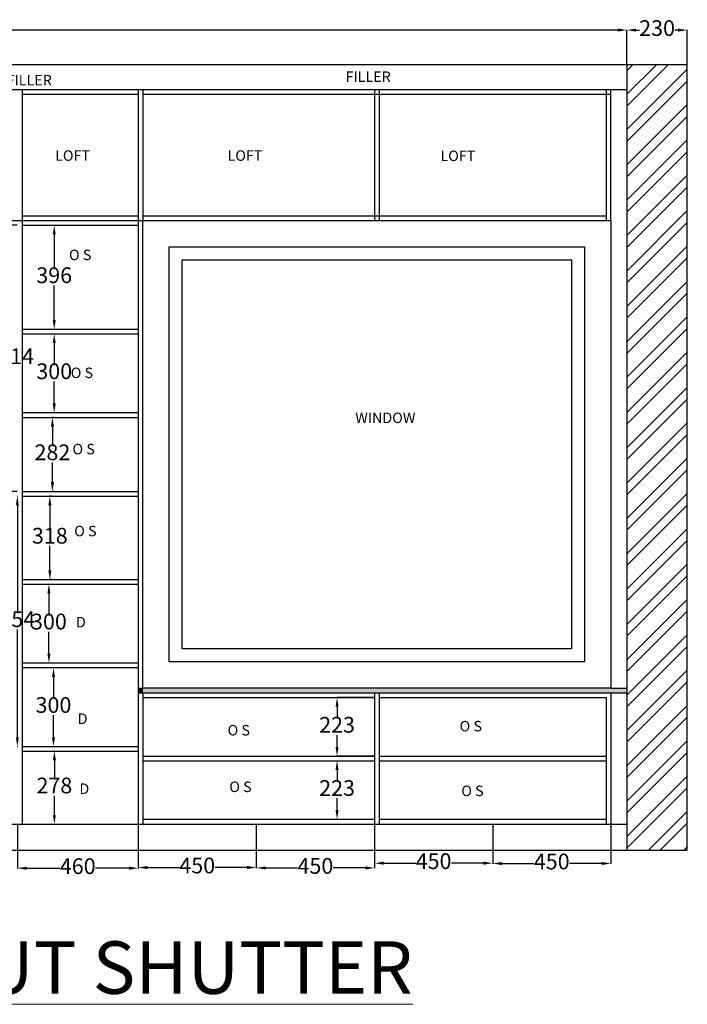
# Model space of a CAD drawing. Units: millimetres. Extents: x 1304 to 14372, y 283 to 7516.
# Tile 3 of 4: x 5077 to 7619, y 283 to 4036. Entities that reach past the tile are written whole.
import ezdxf

# ---------------------------------------------------------------- set-up
doc = ezdxf.new("R2010")
doc.units = ezdxf.units.MM
doc.layers.get('Defpoints').update_dxf_attribs({"color": 2})
for name, color, linetype, lineweight in [('A-ANNO-DIMS', 2, 'Continuous', 18), ('A-ANNO-TEXT', 3, 'Continuous', 18), ('A-FURN', 7, 'Continuous', 25), ('A-FURN-PATT', 8, 'Continuous', 13)]:
    doc.layers.add(name, color=color, linetype=linetype, lineweight=lineweight)
doc.styles.get("Standard").update_dxf_attribs({"font": 'arial.ttf'})
doc.dimstyles.new('ISO-25', dxfattribs={"dimtxt": 60, "dimasz": 35, "dimexe": 1.25, "dimexo": 0.625, "dimtad": 0, "dimtih": 1, "dimtoh": 1, "dimtxsty": 'Standard', "dimcen": 2.5, "dimclrd": 1, "dimclre": 3, "dimadec": 0, "dimazin": 0, "dimtfac": 1, "dimtmove": 0, "dimatfit": 3, "dimfxl": 1, "dimarcsym": 0})

# ---------------------------------------------------------------- blocks, each defined once
blk = doc.blocks.new('*D16')
at = {"layer": 'A-ANNO-DIMS', "color": 0, "lineweight": -2, "transparency": 16777216}
for p, q in [((2248.6, 4008), (2248.6, 3995.4)), ((2283.6, 3996.6), (4728.5, 3996.6)), ((7353.6, 3996.6), (4908.8, 3996.6)), ((7388.6, 3865.9), (7388.6, 3997.9))]:
    blk.add_line(p, q, dxfattribs=at)
at = {"layer": 'A-ANNO-DIMS', "color": 0, "transparency": 16777216}
for points in [[(2283.6, 4002.4), (2283.6, 3990.8), (2248.6, 3996.6)], [(7353.6, 4002.4), (7353.6, 3990.8), (7388.6, 3996.6)]]:
    blk.add_solid(points, dxfattribs=at)
at = {"layer": 'Defpoints', "color": 0, "transparency": 16777216}
for p in [(2248.6, 4008.6), (7388.6, 3996.6), (7388.6, 3865.3)]:
    blk.add_point(p, dxfattribs=at)
at = {"layer": 'A-ANNO-DIMS', "color": 0, "transparency": 16777216, "insert": (4818.6, 3996.6), "char_height": 60, "attachment_point": 5}
blk.add_mtext('5140', dxfattribs=at)
blk = doc.blocks.new('*D17')
at = {"layer": 'A-ANNO-DIMS', "color": 0, "lineweight": -2, "transparency": 16777216}
for p, q in [((7388.6, 3865.9), (7388.6, 3997.5)), ((7423.6, 3996.3), (7436.3, 3996.3)), ((7583.6, 3996.3), (7571, 3996.3)), ((7618.6, 3865.9), (7618.6, 3997.5))]:
    blk.add_line(p, q, dxfattribs=at)
at = {"layer": 'A-ANNO-DIMS', "color": 0, "transparency": 16777216}
for points in [[(7423.6, 4002.1), (7423.6, 3990.4), (7388.6, 3996.3)], [(7583.6, 4002.1), (7583.6, 3990.4), (7618.6, 3996.3)]]:
    blk.add_solid(points, dxfattribs=at)
at = {"layer": 'Defpoints', "color": 0, "transparency": 16777216}
for p in [(7618.6, 3996.3), (7388.6, 3865.3), (7618.6, 3865.3)]:
    blk.add_point(p, dxfattribs=at)
at = {"layer": 'A-ANNO-DIMS', "color": 0, "transparency": 16777216, "insert": (7503.6, 3996.3), "char_height": 60, "attachment_point": 5}
blk.add_mtext('230', dxfattribs=at)
blk = doc.blocks.new('*D23')
at = {"layer": 'A-ANNO-DIMS', "color": 0, "lineweight": -2, "transparency": 16777216}
for p, q in [((5067, 3252.3), (5038.8, 3252.3)), ((5040.1, 3217.3), (5040.1, 2776.5)), ((5040.1, 2273.3), (5040.1, 2714)), ((5067, 2238.3), (5038.8, 2238.3))]:
    blk.add_line(p, q, dxfattribs=at)
at = {"layer": 'A-ANNO-DIMS', "color": 0, "transparency": 16777216}
for points in [[(5034.2, 3217.3), (5045.9, 3217.3), (5040.1, 3252.3)], [(5034.2, 2273.3), (5045.9, 2273.3), (5040.1, 2238.3)]]:
    blk.add_solid(points, dxfattribs=at)
at = {"layer": 'Defpoints', "color": 0, "transparency": 16777216}
for p in [(5067.6, 3252.3), (5040.1, 2238.3), (5067.6, 2238.3)]:
    blk.add_point(p, dxfattribs=at)
at = {"layer": 'A-ANNO-DIMS', "color": 0, "transparency": 16777216, "insert": (5040.1, 2745.3), "char_height": 60, "attachment_point": 5}
blk.add_mtext('1014', dxfattribs=at)
blk = doc.blocks.new('*D24')
at = {"layer": 'A-ANNO-DIMS', "color": 0, "lineweight": -2, "transparency": 16777216}
for p, q in [((5068.3, 2220.3), (5068.9, 2220.3)), ((5067.6, 2185.3), (5067.6, 1774.5)), ((5067.6, 1301.3), (5067.6, 1712)), ((5068.3, 1266.3), (5068.9, 1266.3))]:
    blk.add_line(p, q, dxfattribs=at)
at = {"layer": 'A-ANNO-DIMS', "color": 0, "transparency": 16777216}
for points in [[(5061.8, 2185.3), (5073.5, 2185.3), (5067.6, 2220.3)], [(5061.8, 1301.3), (5073.5, 1301.3), (5067.6, 1266.3)]]:
    blk.add_solid(points, dxfattribs=at)
at = {"layer": 'Defpoints', "color": 0, "transparency": 16777216}
for p in [(5067.6, 2220.3), (5067.6, 1266.3), (5067.6, 1266.3)]:
    blk.add_point(p, dxfattribs=at)
at = {"layer": 'A-ANNO-DIMS', "color": 0, "transparency": 16777216, "insert": (5067.6, 1743.3), "char_height": 60, "attachment_point": 5}
blk.add_mtext('954', dxfattribs=at)
blk = doc.blocks.new('*D25')
at = {"layer": 'A-ANNO-DIMS', "color": 0, "lineweight": -2, "transparency": 16777216}
for p, q in [((5086.3, 3252.3), (5209.4, 3252.3)), ((5208.1, 3217.3), (5208.1, 3085.6)), ((5208.1, 2891.3), (5208.1, 3023)), ((5086.3, 2856.3), (5209.4, 2856.3))]:
    blk.add_line(p, q, dxfattribs=at)
at = {"layer": 'A-ANNO-DIMS', "color": 0, "transparency": 16777216}
for points in [[(5202.3, 3217.3), (5213.9, 3217.3), (5208.1, 3252.3)], [(5202.3, 2891.3), (5213.9, 2891.3), (5208.1, 2856.3)]]:
    blk.add_solid(points, dxfattribs=at)
at = {"layer": 'Defpoints', "color": 0, "transparency": 16777216}
for p in [(5085.6, 3252.3), (5085.6, 2856.3), (5208.1, 2856.3)]:
    blk.add_point(p, dxfattribs=at)
at = {"layer": 'A-ANNO-DIMS', "color": 0, "transparency": 16777216, "insert": (5208.1, 3054.3), "char_height": 60, "attachment_point": 5}
blk.add_mtext('396', dxfattribs=at)
blk = doc.blocks.new('*D26')
at = {"layer": 'A-ANNO-DIMS', "color": 0, "lineweight": -2, "transparency": 16777216}
for p, q in [((5208.7, 2838.3), (5209.4, 2838.3)), ((5208.1, 2803.3), (5208.1, 2719.6)), ((5208.1, 2573.3), (5208.1, 2657)), ((5208.7, 2538.3), (5209.4, 2538.3))]:
    blk.add_line(p, q, dxfattribs=at)
at = {"layer": 'A-ANNO-DIMS', "color": 0, "transparency": 16777216}
for points in [[(5202.3, 2803.3), (5213.9, 2803.3), (5208.1, 2838.3)], [(5202.3, 2573.3), (5213.9, 2573.3), (5208.1, 2538.3)]]:
    blk.add_solid(points, dxfattribs=at)
at = {"layer": 'Defpoints', "color": 0, "transparency": 16777216}
for p in [(5208.1, 2838.3), (5208.1, 2538.3), (5208.1, 2538.3)]:
    blk.add_point(p, dxfattribs=at)
at = {"layer": 'A-ANNO-DIMS', "color": 0, "transparency": 16777216, "insert": (5208.1, 2688.3), "char_height": 60, "attachment_point": 5}
blk.add_mtext('300', dxfattribs=at)
blk = doc.blocks.new('*D27')
at = {"layer": 'A-ANNO-DIMS', "color": 0, "lineweight": -2, "transparency": 16777216}
for p, q in [((5207.5, 2520.3), (5199.9, 2520.3)), ((5201.2, 2485.3), (5201.2, 2410.5)), ((5201.2, 2273.3), (5201.2, 2348)), ((5207.5, 2238.3), (5199.9, 2238.3))]:
    blk.add_line(p, q, dxfattribs=at)
at = {"layer": 'A-ANNO-DIMS', "color": 0, "transparency": 16777216}
for points in [[(5195.4, 2485.3), (5207, 2485.3), (5201.2, 2520.3)], [(5195.4, 2273.3), (5207, 2273.3), (5201.2, 2238.3)]]:
    blk.add_solid(points, dxfattribs=at)
at = {"layer": 'Defpoints', "color": 0, "transparency": 16777216}
for p in [(5208.1, 2520.3), (5201.2, 2238.3), (5208.1, 2238.3)]:
    blk.add_point(p, dxfattribs=at)
at = {"layer": 'A-ANNO-DIMS', "color": 0, "transparency": 16777216, "insert": (5201.2, 2379.3), "char_height": 60, "attachment_point": 5}
blk.add_mtext('282', dxfattribs=at)
blk = doc.blocks.new('*D28')
at = {"layer": 'A-ANNO-DIMS', "color": 0, "lineweight": -2, "transparency": 16777216}
for p, q in [((5200.6, 2220.3), (5190.2, 2220.3)), ((5191.4, 2185.3), (5191.4, 2092.6)), ((5191.4, 1937.3), (5191.4, 2030)), ((5200.6, 1902.3), (5190.2, 1902.3))]:
    blk.add_line(p, q, dxfattribs=at)
at = {"layer": 'A-ANNO-DIMS', "color": 0, "transparency": 16777216}
for points in [[(5185.6, 2185.3), (5197.3, 2185.3), (5191.4, 2220.3)], [(5185.6, 1937.3), (5197.3, 1937.3), (5191.4, 1902.3)]]:
    blk.add_solid(points, dxfattribs=at)
at = {"layer": 'Defpoints', "color": 0, "transparency": 16777216}
for p in [(5201.2, 2220.3), (5191.4, 1902.3), (5201.2, 1902.3)]:
    blk.add_point(p, dxfattribs=at)
at = {"layer": 'A-ANNO-DIMS', "color": 0, "transparency": 16777216, "insert": (5191.4, 2061.3), "char_height": 60, "attachment_point": 5}
blk.add_mtext('318', dxfattribs=at)
blk = doc.blocks.new('*D29')
at = {"layer": 'A-ANNO-DIMS', "color": 0, "lineweight": -2, "transparency": 16777216}
for p, q in [((5205.8, 1566.3), (5206.4, 1566.3)), ((5205.2, 1531.3), (5205.2, 1447.6)), ((5205.2, 1301.3), (5205.2, 1385)), ((5205.8, 1266.3), (5206.4, 1266.3))]:
    blk.add_line(p, q, dxfattribs=at)
at = {"layer": 'A-ANNO-DIMS', "color": 0, "transparency": 16777216}
for points in [[(5199.4, 1531.3), (5211, 1531.3), (5205.2, 1566.3)], [(5199.4, 1301.3), (5211, 1301.3), (5205.2, 1266.3)]]:
    blk.add_solid(points, dxfattribs=at)
at = {"layer": 'Defpoints', "color": 0, "transparency": 16777216}
for p in [(5205.2, 1566.3), (5205.2, 1266.3), (5205.2, 1266.3)]:
    blk.add_point(p, dxfattribs=at)
at = {"layer": 'A-ANNO-DIMS', "color": 0, "transparency": 16777216, "insert": (5205.2, 1416.3), "char_height": 60, "attachment_point": 5}
blk.add_mtext('300', dxfattribs=at)
blk = doc.blocks.new('*D30')
at = {"layer": 'A-ANNO-DIMS', "color": 0, "lineweight": -2, "transparency": 16777216}
for p, q in [((5205.8, 1248.3), (5209.9, 1248.3)), ((5208.6, 1213.3), (5208.6, 1140.5)), ((5208.6, 1005.3), (5208.6, 1078)), ((5205.8, 970.3), (5209.9, 970.3))]:
    blk.add_line(p, q, dxfattribs=at)
at = {"layer": 'A-ANNO-DIMS', "color": 0, "transparency": 16777216}
for points in [[(5202.8, 1213.3), (5214.5, 1213.3), (5208.6, 1248.3)], [(5202.8, 1005.3), (5214.5, 1005.3), (5208.6, 970.3)]]:
    blk.add_solid(points, dxfattribs=at)
at = {"layer": 'Defpoints', "color": 0, "transparency": 16777216}
for p in [(5205.2, 1248.3), (5205.2, 970.3), (5208.6, 970.3)]:
    blk.add_point(p, dxfattribs=at)
at = {"layer": 'A-ANNO-DIMS', "color": 0, "transparency": 16777216, "insert": (5208.6, 1109.3), "char_height": 60, "attachment_point": 5}
blk.add_mtext('278', dxfattribs=at)
blk = doc.blocks.new('*D31')
at = {"layer": 'A-ANNO-DIMS', "color": 0, "lineweight": -2, "transparency": 16777216}
for p, q in [((6427, 1452.3), (6283.8, 1452.3)), ((6285, 1417.3), (6285, 1372.1)), ((6285, 1264.3), (6285, 1309.5)), ((6427, 1229.3), (6283.8, 1229.3))]:
    blk.add_line(p, q, dxfattribs=at)
at = {"layer": 'A-ANNO-DIMS', "color": 0, "transparency": 16777216}
for points in [[(6279.2, 1417.3), (6290.9, 1417.3), (6285, 1452.3)], [(6279.2, 1264.3), (6290.9, 1264.3), (6285, 1229.3)]]:
    blk.add_solid(points, dxfattribs=at)
at = {"layer": 'Defpoints', "color": 0, "transparency": 16777216}
for p in [(6427.6, 1452.3), (6285, 1229.3), (6427.6, 1229.3)]:
    blk.add_point(p, dxfattribs=at)
at = {"layer": 'A-ANNO-DIMS', "color": 0, "transparency": 16777216, "insert": (6285, 1340.8), "char_height": 60, "attachment_point": 5}
blk.add_mtext('223', dxfattribs=at)
blk = doc.blocks.new('*D32')
at = {"layer": 'A-ANNO-DIMS', "color": 0, "lineweight": -2, "transparency": 16777216}
for p, q in [((6285.7, 1211.3), (6286.3, 1211.3)), ((6285, 1176.3), (6285, 1131.1)), ((6285, 1023.3), (6285, 1068.5)), ((6285.7, 988.3), (6286.3, 988.3))]:
    blk.add_line(p, q, dxfattribs=at)
at = {"layer": 'A-ANNO-DIMS', "color": 0, "transparency": 16777216}
for points in [[(6279.2, 1176.3), (6290.9, 1176.3), (6285, 1211.3)], [(6279.2, 1023.3), (6290.9, 1023.3), (6285, 988.3)]]:
    blk.add_solid(points, dxfattribs=at)
at = {"layer": 'Defpoints', "color": 0, "transparency": 16777216}
for p in [(6285, 1211.3), (6285, 988.3), (6285, 988.3)]:
    blk.add_point(p, dxfattribs=at)
at = {"layer": 'A-ANNO-DIMS', "color": 0, "transparency": 16777216, "insert": (6285, 1099.8), "char_height": 60, "attachment_point": 5}
blk.add_mtext('223', dxfattribs=at)
blk = doc.blocks.new('*D39')
at = {"layer": 'A-ANNO-DIMS', "color": 0, "lineweight": -2, "transparency": 16777216}
for p, q in [((5067.6, 969.7), (5067.6, 800.7)), ((5527.6, 969.7), (5527.6, 800.7)), ((5102.6, 802), (5229.6, 802)), ((5492.6, 802), (5365.7, 802))]:
    blk.add_line(p, q, dxfattribs=at)
at = {"layer": 'A-ANNO-DIMS', "color": 0, "transparency": 16777216}
for points in [[(5102.6, 807.8), (5102.6, 796.1), (5067.6, 802)], [(5492.6, 807.8), (5492.6, 796.1), (5527.6, 802)]]:
    blk.add_solid(points, dxfattribs=at)
at = {"layer": 'Defpoints', "color": 0, "transparency": 16777216}
for p in [(5067.6, 970.3), (5527.6, 970.3), (5527.6, 802)]:
    blk.add_point(p, dxfattribs=at)
at = {"layer": 'A-ANNO-DIMS', "color": 0, "transparency": 16777216, "insert": (5297.6, 802), "char_height": 60, "attachment_point": 5}
blk.add_mtext('460', dxfattribs=at)
blk = doc.blocks.new('*D40')
at = {"layer": 'A-ANNO-DIMS', "color": 0, "lineweight": -2, "transparency": 16777216}
for p, q in [((5527.6, 969.7), (5527.6, 803.3)), ((5977.6, 969.7), (5977.6, 803.3)), ((5562.6, 804.5), (5684.6, 804.5)), ((5942.6, 804.5), (5820.7, 804.5))]:
    blk.add_line(p, q, dxfattribs=at)
at = {"layer": 'A-ANNO-DIMS', "color": 0, "transparency": 16777216}
for points in [[(5562.6, 810.4), (5562.6, 798.7), (5527.6, 804.5)], [(5942.6, 810.4), (5942.6, 798.7), (5977.6, 804.5)]]:
    blk.add_solid(points, dxfattribs=at)
at = {"layer": 'Defpoints', "color": 0, "transparency": 16777216}
for p in [(5527.6, 970.3), (5977.6, 970.3), (5977.6, 804.5)]:
    blk.add_point(p, dxfattribs=at)
at = {"layer": 'A-ANNO-DIMS', "color": 0, "transparency": 16777216, "insert": (5752.6, 804.5), "char_height": 60, "attachment_point": 5}
blk.add_mtext('450', dxfattribs=at)
blk = doc.blocks.new('*D41')
at = {"layer": 'A-ANNO-DIMS', "color": 0, "lineweight": -2, "transparency": 16777216}
for p, q in [((5977.6, 969.7), (5977.6, 801.8)), ((6427.6, 969.7), (6427.6, 801.8)), ((6012.6, 803), (6134.6, 803)), ((6392.6, 803), (6270.7, 803))]:
    blk.add_line(p, q, dxfattribs=at)
at = {"layer": 'A-ANNO-DIMS', "color": 0, "transparency": 16777216}
for points in [[(6012.6, 808.8), (6012.6, 797.2), (5977.6, 803)], [(6392.6, 808.8), (6392.6, 797.2), (6427.6, 803)]]:
    blk.add_solid(points, dxfattribs=at)
at = {"layer": 'Defpoints', "color": 0, "transparency": 16777216}
for p in [(5977.6, 970.3), (6427.6, 970.3), (6427.6, 803)]:
    blk.add_point(p, dxfattribs=at)
at = {"layer": 'A-ANNO-DIMS', "color": 0, "transparency": 16777216, "insert": (6202.6, 803), "char_height": 60, "attachment_point": 5}
blk.add_mtext('450', dxfattribs=at)
blk = doc.blocks.new('*D42')
at = {"layer": 'A-ANNO-DIMS', "color": 0, "lineweight": -2, "transparency": 16777216}
for p, q in [((6427.6, 969.7), (6427.6, 819.9)), ((6877.6, 969.7), (6877.6, 819.9)), ((6462.6, 821.1), (6584.6, 821.1)), ((6842.6, 821.1), (6720.7, 821.1))]:
    blk.add_line(p, q, dxfattribs=at)
at = {"layer": 'A-ANNO-DIMS', "color": 0, "transparency": 16777216}
for points in [[(6462.6, 827), (6462.6, 815.3), (6427.6, 821.1)], [(6842.6, 827), (6842.6, 815.3), (6877.6, 821.1)]]:
    blk.add_solid(points, dxfattribs=at)
at = {"layer": 'Defpoints', "color": 0, "transparency": 16777216}
for p in [(6427.6, 970.3), (6877.6, 970.3), (6877.6, 821.1)]:
    blk.add_point(p, dxfattribs=at)
at = {"layer": 'A-ANNO-DIMS', "color": 0, "transparency": 16777216, "insert": (6652.6, 821.1), "char_height": 60, "attachment_point": 5}
blk.add_mtext('450', dxfattribs=at)
blk = doc.blocks.new('*D43')
at = {"layer": 'A-ANNO-DIMS', "color": 0, "lineweight": -2, "transparency": 16777216}
for p, q in [((6877.6, 969.7), (6877.6, 818.7)), ((7327.6, 969.7), (7327.6, 818.7)), ((6912.6, 819.9), (7034.6, 819.9)), ((7292.6, 819.9), (7170.7, 819.9))]:
    blk.add_line(p, q, dxfattribs=at)
at = {"layer": 'A-ANNO-DIMS', "color": 0, "transparency": 16777216}
for points in [[(6912.6, 825.8), (6912.6, 814.1), (6877.6, 819.9)], [(7292.6, 825.8), (7292.6, 814.1), (7327.6, 819.9)]]:
    blk.add_solid(points, dxfattribs=at)
at = {"layer": 'Defpoints', "color": 0, "transparency": 16777216}
for p in [(6877.6, 970.3), (7327.6, 970.3), (7327.6, 819.9)]:
    blk.add_point(p, dxfattribs=at)
at = {"layer": 'A-ANNO-DIMS', "color": 0, "transparency": 16777216, "insert": (7102.6, 819.9), "char_height": 60, "attachment_point": 5}
blk.add_mtext('450', dxfattribs=at)
blk = doc.blocks.new('*D45')
at = {"layer": 'A-ANNO-DIMS', "color": 0, "lineweight": -2, "transparency": 16777216}
for p, q in [((5086.3, 1884.3), (5189.1, 1884.3)), ((5187.9, 1849.3), (5187.9, 1765.6)), ((5187.9, 1619.3), (5187.9, 1703)), ((5086.3, 1584.3), (5189.1, 1584.3))]:
    blk.add_line(p, q, dxfattribs=at)
at = {"layer": 'A-ANNO-DIMS', "color": 0, "transparency": 16777216}
for points in [[(5182, 1849.3), (5193.7, 1849.3), (5187.9, 1884.3)], [(5182, 1619.3), (5193.7, 1619.3), (5187.9, 1584.3)]]:
    blk.add_solid(points, dxfattribs=at)
at = {"layer": 'Defpoints', "color": 0, "transparency": 16777216}
for p in [(5085.6, 1884.3), (5085.6, 1584.3), (5187.9, 1584.3)]:
    blk.add_point(p, dxfattribs=at)
at = {"layer": 'A-ANNO-DIMS', "color": 0, "transparency": 16777216, "insert": (5187.9, 1734.3), "char_height": 60, "attachment_point": 5}
blk.add_mtext('300', dxfattribs=at)

msp = doc.modelspace()

# ---------------------------------------------------------------- hatches: boundary and pattern name
at = {"layer": 'A-FURN-PATT'}
h = msp.add_hatch(dxfattribs=at)
h.set_pattern_fill('ANSI32', color=256, scale=10)
h.paths.add_polyline_path([(2018.643, 870.285), (2248.643, 870.285), (2248.643, 3865.285), (2018.643, 3865.285)])
h.paths.add_polyline_path([(7388.643, 870.285), (7618.643, 870.285), (7618.643, 3865.285), (7388.643, 3865.285)])
h = msp.add_hatch(color=256, dxfattribs=at)
h.dxf.hatch_style = 1
h.paths.add_polyline_path([(5545.643, 1488.285), (5527.643, 1488.285), (5527.643, 1470.285), (5545.643, 1470.285)])
h = msp.add_hatch(color=256, dxfattribs=at)
h.dxf.hatch_style = 1
h.paths.add_polyline_path([(7388.643, 1488.285), (7327.643, 1488.285), (5545.643, 1488.285), (5527.643, 1488.285), (5527.643, 1470.285), (7388.643, 1470.285)])

# ---------------------------------------------------------------- linework, layer by layer
at = {"layer": 'A-FURN'}
for p, q in [((2018.643, 3865.285), (7618.643, 3865.285)), ((7388.643, 3865.285), (7388.643, 870.285)), ((7618.643, 870.285), (7618.643, 3865.285)), ((2316.643, 3770.285), (7388.643, 3770.285)), ((5085.643, 3770.285), (5085.643, 970.285)), ((5527.643, 3770.285), (5527.643, 1470.285)), ((5545.643, 3770.285), (5545.643, 3270.285)), ((6427.643, 3770.285), (6427.643, 3270.285)), ((6445.643, 3770.285), (6445.643, 3270.285)), ((7309.643, 3770.285), (7309.643, 3270.285)), ((5085.643, 3752.285), (5527.643, 3752.285)), ((5545.643, 3752.285), (7327.643, 3752.285)), ((2316.643, 3270.285), (5545.643, 3270.285)), ((5085.643, 3288.285), (5527.643, 3288.285)), ((5545.643, 3288.285), (7309.643, 3288.285)), ((5085.643, 3252.285), (5527.643, 3252.285)), ((5085.643, 2856.285), (5527.643, 2856.285)), ((5085.643, 2838.285), (5527.643, 2838.285)), ((5085.643, 2538.285), (5527.643, 2538.285)), ((5085.643, 2520.285), (5527.643, 2520.285)), ((5085.643, 2238.285), (5527.643, 2238.285)), ((5085.643, 2220.285), (5527.643, 2220.285)), ((5085.643, 1902.285), (5527.643, 1902.285)), ((5085.643, 1884.285), (5527.643, 1884.285)), ((5085.643, 1584.285), (5527.643, 1584.285)), ((5085.643, 1566.285), (5527.643, 1566.285)), ((5527.643, 1488.285), (5545.643, 1488.285)), ((5527.643, 1470.285), (7388.643, 1470.285)), ((5527.643, 1470.285), (5527.643, 970.285)), ((5545.643, 1470.285), (5545.643, 970.285)), ((6427.643, 1470.285), (6427.643, 970.285)), ((6445.643, 1470.285), (6445.643, 970.285)), ((7327.643, 1488.285), (7388.643, 1488.285)), ((7327.643, 1470.285), (7327.643, 970.285)), ((5545.643, 1452.285), (6427.643, 1452.285)), ((6445.643, 1452.285), (7309.643, 1452.285)), ((7309.643, 1452.285), (7309.643, 970.285)), ((5085.643, 1266.285), (5527.643, 1266.285)), ((5085.643, 1248.285), (5527.643, 1248.285)), ((5545.643, 1229.285), (6427.643, 1229.285)), ((5545.643, 1211.285), (6427.643, 1211.285)), ((6445.643, 1229.285), (7309.643, 1229.285)), ((6445.643, 1211.285), (7309.643, 1211.285)), ((5545.643, 988.285), (6427.643, 988.285)), ((6445.643, 988.285), (7309.643, 988.285)), ((4147.643, 970.285), (5527.643, 970.285)), ((5527.643, 970.285), (7388.643, 970.285)), ((2018.643, 870.285), (7618.643, 870.285))]:
    msp.add_line(p, q, dxfattribs=at)
msp.add_lwpolyline([(7327.643, 3270.285), (7327.643, 3770.285)], dxfattribs=at)
for points in [[(5545.643, 1488.285), (5545.643, 3270.285), (7327.643, 3270.285), (7327.643, 1488.285)], [(5645.643, 1588.285), (5645.643, 3170.285), (7227.643, 3170.285), (7227.643, 1588.285)], [(5695.643, 1638.285), (5695.643, 3120.285), (7177.643, 3120.285), (7177.643, 1638.285)]]:
    msp.add_lwpolyline(points, close=True, dxfattribs=at)

# ---------------------------------------------------------------- texts
at = {"layer": 'A-ANNO-TEXT', "attachment_point": 1}
for s, width, gutter_width, insert, char_height in [('FILLER', 605.86509, 50, (6317.313, 3838.722), 40), ('FILLER', 605.86509, 50, (5026.806, 3825.394), 40), ('LOFT', 605.86509, 50, (5211.426, 3538.046), 40), ('LOFT', 605.86509, 50, (5868.014, 3538.046), 40), ('LOFT', 605.86509, 50, (6678.645, 3537.2), 40), ('O S', 605.86509, 50, (5264.436, 3159.561), 40), ('O S', 605.86509, 50, (5271.01, 2709.962), 40), ('WINDOW', 605.86509, 50, (6354.265, 2538.564), 40), ('O S', 605.86509, 50, (5277.584, 2419.255), 40), ('O S', 605.86509, 50, (5284.159, 2106.933), 40), ('D', 605.86509, 50, (5290.733, 1759.571), 40), ('D', 605.86509, 50, (5297.307, 1391.738), 40), ('O S', 605.86509, 50, (6751.608, 1363.373), 40), ('O S', 605.86509, 50, (5868.195, 1347.96), 40), ('O S', 605.86509, 50, (5874.769, 1132.188), 40), ('D', 605.86509, 50, (5303.881, 1124.932), 40), ('O S', 605.86509, 50, (6758.182, 1116.775), 40), ('{\\LELEVATION WITHOUT SHUTTER}', 5143.98189, 100, (2552.356, 523.2), 200)]:
    msp.add_mtext_dynamic_manual_height_columns(s, width=width, gutter_width=gutter_width, heights=[0], dxfattribs=dict(at, insert=insert, char_height=char_height))

# ---------------------------------------------------------------- dimensions: what is measured, and where the dimension line sits
at = {"layer": 'A-ANNO-DIMS'}
for base, p1, p2, picture, middle in [((7388.643, 3996.603), (2248.643, 4008.602), (7388.643, 3865.285), '*D16', (4818.643, 3996.603)), ((7618.643, 3996.256), (7388.643, 3865.285), (7618.643, 3865.285), '*D17', (7503.643, 3996.256)), ((5527.643, 801.959), (5067.643, 970.285), (5527.643, 970.285), '*D39', (5297.643, 801.959)), ((5977.643, 804.537), (5527.643, 970.285), (5977.643, 970.285), '*D40', (5752.643, 804.537)), ((6427.643, 803.003), (5977.643, 970.285), (6427.643, 970.285), '*D41', (6202.643, 803.003)), ((6877.643, 821.131), (6427.643, 970.285), (6877.643, 970.285), '*D42', (6652.643, 821.131)), ((7327.643, 819.945), (6877.643, 970.285), (7327.643, 970.285), '*D43', (7102.643, 819.945))]:
    dim = msp.add_linear_dim(base=base, p1=p1, p2=p2, dimstyle='ISO-25', override={"dimclrd": 0, "dimclre": 0, "dimclrt": 0}, dxfattribs=at)
    dim.commit()
    dim.dimension.update_dxf_attribs({"geometry": picture, "text_midpoint": middle})
for base, p1, p2, picture, middle in [((5040.059, 2238.285), (5067.643, 3252.285), (5067.643, 2238.285), '*D23', (5040.059, 2745.285)), ((5208.111, 2856.285), (5085.643, 3252.285), (5085.643, 2856.285), '*D25', (5208.111, 3054.285)), ((5208.111, 2538.285), (5208.111, 2838.285), (5208.111, 2538.285), '*D26', (5208.111, 2688.285)), ((5201.198, 2238.285), (5208.111, 2520.285), (5208.111, 2238.285), '*D27', (5201.198, 2379.285)), ((5067.643, 1266.285), (5067.643, 2220.285), (5067.643, 1266.285), '*D24', (5067.643, 1743.285)), ((5191.442, 1902.285), (5201.198, 2220.285), (5201.198, 1902.285), '*D28', (5191.442, 2061.285)), ((5187.879, 1584.285), (5085.643, 1884.285), (5085.643, 1584.285), '*D45', (5187.879, 1734.285)), ((5205.198, 1266.285), (5205.198, 1566.285), (5205.198, 1266.285), '*D29', (5205.198, 1416.285)), ((6285.037, 1229.285), (6427.643, 1452.285), (6427.643, 1229.285), '*D31', (6285.037, 1340.785)), ((5208.637, 970.285), (5205.198, 1248.285), (5205.198, 970.285), '*D30', (5208.637, 1109.285)), ((6285.037, 988.285), (6285.037, 1211.285), (6285.037, 988.285), '*D32', (6285.037, 1099.785))]:
    dim = msp.add_linear_dim(base=base, p1=p1, p2=p2, angle=90, dimstyle='ISO-25', override={"dimclrd": 0, "dimclre": 0, "dimclrt": 0}, dxfattribs=at)
    dim.commit()
    dim.dimension.update_dxf_attribs({"geometry": picture, "text_midpoint": middle})

doc.saveas('drawing.dxf')
